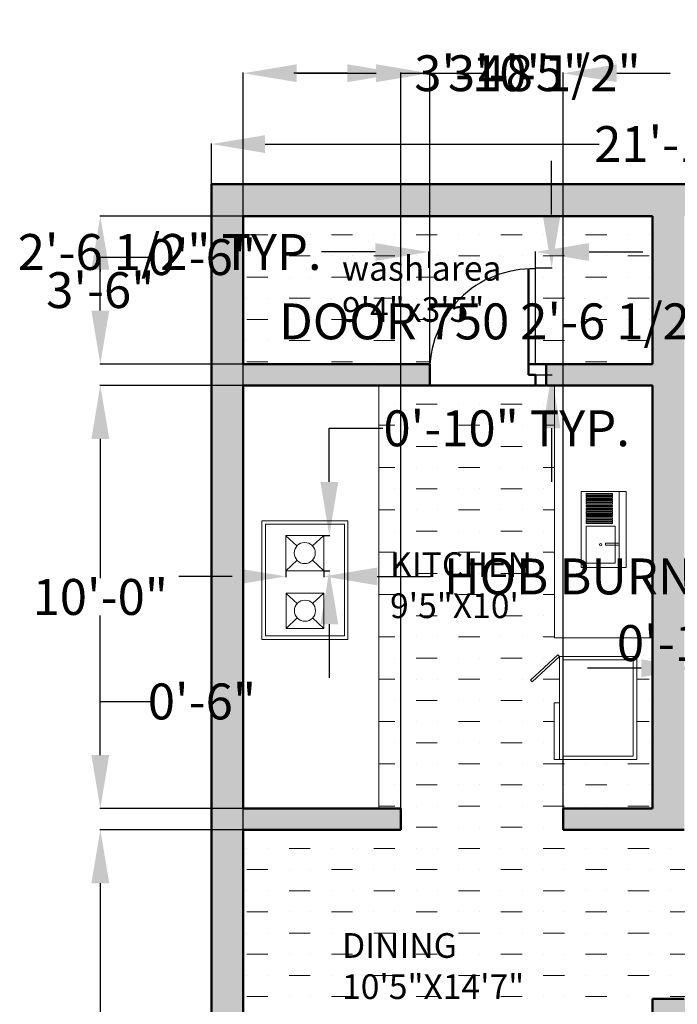
# Model space of a CAD drawing. Units: inches. Extents: x 26 to 14419, y 2 to 3479.
# Tile 4 of 9: x 13605 to 13791, y 3199 to 3479. Entities that reach past the tile are written whole.
import ezdxf

# ---------------------------------------------------------------- set-up
doc = ezdxf.new("R2010")
doc.units = ezdxf.units.IN
doc.header["$MEASUREMENT"] = 0
for name, color, linetype, lineweight in [('A-ANNO-DIMS', 2, 'Continuous', 18), ('A-AREA-IDEN', 7, 'Continuous', 18), ('A-DOOR', 4, 'Continuous', 25), ('A-FLOR-FIXT', 8, 'Continuous', 18), ('A-FLOR-PATT', 252, 'Continuous', 13), ('A-FURN', 8, 'Continuous', 18), ('A-WALL', 7, 'Continuous', 50)]:
    doc.layers.add(name, color=color, linetype=linetype, lineweight=lineweight)
doc.styles.get("Standard").update_dxf_attribs({"font": 'arial.ttf'})
doc.dimstyles.get("Standard").update_dxf_attribs({"dimtxt": 10.18, "dimasz": 15.18, "dimexe": 0.18, "dimexo": 0.0625, "dimgap": 0.09, "dimtad": 0, "dimtih": 1, "dimtoh": 1, "dimdec": 0, "dimzin": 0, "dimdsep": 46, "dimlunit": 3, "dimtxsty": 'Standard', "dimcen": 0.09, "dimadec": 0, "dimazin": 0, "dimtfac": 1, "dimtdec": 0, "dimtofl": 0, "dimtmove": 0, "dimatfit": 3, "dimfxl": 1, "dimtolj": 1, "dimtzin": 0, "dimarcsym": 0})
pattern_1 = [(0, (61.093, 57.669), (12, 6), [6, -6, 0, -6, 0, -6])]

# ---------------------------------------------------------------- blocks, each defined once
blk = doc.blocks.new('*D6')
at = {"layer": 'A-ANNO-DIMS', "color": 0, "lineweight": -2, "transparency": 16777216}
for p, q in [((13659.09, 3432.06), (13659.09, 3443.59)), ((13674.27, 3443.41), (13768.97, 3443.41)), ((13906.91, 3443.41), (13812.21, 3443.41)), ((13922.09, 3432.06), (13922.09, 3443.59))]:
    blk.add_line(p, q, dxfattribs=at)
at = {"layer": 'A-ANNO-DIMS', "color": 0, "transparency": 16777216}
for points in [[(13674.27, 3445.94), (13674.27, 3440.88), (13659.09, 3443.41)], [(13906.91, 3445.94), (13906.91, 3440.88), (13922.09, 3443.41)]]:
    blk.add_solid(points, dxfattribs=at)
at = {"layer": 'Defpoints', "color": 0, "transparency": 16777216}
for p in [(13922.09, 3443.41), (13659.09, 3432), (13922.09, 3432)]:
    blk.add_point(p, dxfattribs=at)
at = {"layer": 'A-ANNO-DIMS', "color": 0, "transparency": 16777216, "insert": (13790.59, 3443.41), "char_height": 10.18, "attachment_point": 5}
blk.add_mtext('\\A1;21\'-11"', dxfattribs=at)
blk = doc.blocks.new('DOOR-750')
blk.add_line((3, 0), (30, 0))
blk.add_arc((1, 1), 29.02, 358.0251, 91.9749)
blk = doc.blocks.new('HOB-BURNER')
for p, q in [((0, 9.87), (3.14, 7.02)), ((10.72, 10.03), (7.54, 7.06)), ((0, 0), (3.17, 2.97)), ((10.72, 0), (7.54, 2.97))]:
    blk.add_line(p, q)
blk.add_lwpolyline([(0, 10.03), (10.72, 10.03), (10.72, 0), (0, 0)], close=True)
blk.add_circle((5.36, 5.02), 2.99)
blk = doc.blocks.new('*D24')
at = {"layer": 'A-ANNO-DIMS', "color": 0, "lineweight": -2, "transparency": 16777216}
for p, q in [((13730.53, 3172.73), (13730.53, 3187.91)), ((13730.53, 3187.91), (13745.71, 3187.91)), ((13728.71, 3157.55), (13730.71, 3157.55)), ((13728.71, 3147.87), (13730.71, 3147.87)), ((13730.53, 3132.69), (13730.53, 3117.51))]:
    blk.add_line(p, q, dxfattribs=at)
at = {"layer": 'A-ANNO-DIMS', "color": 0, "transparency": 16777216}
for points in [[(13728, 3172.73), (13733.06, 3172.73), (13730.53, 3157.55)], [(13728, 3132.69), (13733.06, 3132.69), (13730.53, 3147.87)]]:
    blk.add_solid(points, dxfattribs=at)
at = {"layer": 'Defpoints', "color": 0, "transparency": 16777216}
for p in [(13728.65, 3157.55), (13730.53, 3157.55), (13728.65, 3147.87)]:
    blk.add_point(p, dxfattribs=at)
at = {"layer": 'A-ANNO-DIMS', "color": 0, "transparency": 16777216, "insert": (13788.69, 3187.91), "char_height": 10.18, "attachment_point": 5}
blk.add_mtext('\\A1;0\'-9 1/2" TYP.', dxfattribs=at)
blk = doc.blocks.new('*D27')
at = {"layer": 'A-ANNO-DIMS', "color": 0, "lineweight": -2, "transparency": 16777216}
for p, q in [((13755.48, 3423.45), (13755.48, 3438.63)), ((13751.01, 3408.27), (13755.66, 3408.27)), ((13751.01, 3378), (13755.66, 3378)), ((13755.48, 3362.82), (13755.48, 3347.64))]:
    blk.add_line(p, q, dxfattribs=at)
at = {"layer": 'A-ANNO-DIMS', "color": 0, "transparency": 16777216}
for points in [[(13752.95, 3423.45), (13758.01, 3423.45), (13755.48, 3408.27)], [(13752.95, 3362.82), (13758.01, 3362.82), (13755.48, 3378)]]:
    blk.add_solid(points, dxfattribs=at)
at = {"layer": 'Defpoints', "color": 0, "transparency": 16777216}
for p in [(13750.94, 3408.27), (13755.48, 3408.27), (13750.94, 3378)]:
    blk.add_point(p, dxfattribs=at)
at = {"layer": 'A-ANNO-DIMS', "color": 0, "transparency": 16777216, "insert": (13755.48, 3393.13), "char_height": 10.18, "attachment_point": 5}
blk.add_mtext('\\A1;DOOR 750 2\'-6 1/2" TYP.', dxfattribs=at)
blk = doc.blocks.new('*D28')
at = {"layer": 'A-ANNO-DIMS', "color": 0, "lineweight": -2, "transparency": 16777216}
for p, q in [((13705.49, 3412.81), (13690.31, 3412.81)), ((13720.67, 3408.34), (13720.67, 3412.99)), ((13750.94, 3408.34), (13750.94, 3412.99)), ((13766.12, 3412.81), (13781.3, 3412.81))]:
    blk.add_line(p, q, dxfattribs=at)
at = {"layer": 'A-ANNO-DIMS', "color": 0, "transparency": 16777216}
for points in [[(13705.49, 3415.34), (13705.49, 3410.28), (13720.67, 3412.81)], [(13766.12, 3415.34), (13766.12, 3410.28), (13750.94, 3412.81)]]:
    blk.add_solid(points, dxfattribs=at)
at = {"layer": 'Defpoints', "color": 0, "transparency": 16777216}
for p in [(13720.67, 3412.81), (13720.67, 3408.27), (13750.94, 3408.27)]:
    blk.add_point(p, dxfattribs=at)
at = {"layer": 'A-ANNO-DIMS', "color": 0, "transparency": 16777216, "insert": (13647.24, 3412.81), "char_height": 10.18, "attachment_point": 5}
blk.add_mtext('\\A1;2\'-6 1/2" TYP.', dxfattribs=at)
blk = doc.blocks.new('*D35')
at = {"layer": 'A-ANNO-DIMS', "color": 0, "lineweight": -2, "transparency": 16777216}
for p, q in [((13780.88, 3294.79), (13765.7, 3294.79)), ((13796.06, 3296.4), (13796.06, 3294.61)), ((13807.24, 3296.4), (13807.24, 3294.61)), ((13822.42, 3294.79), (13837.6, 3294.79))]:
    blk.add_line(p, q, dxfattribs=at)
at = {"layer": 'A-ANNO-DIMS', "color": 0, "transparency": 16777216}
for points in [[(13780.88, 3297.32), (13780.88, 3292.26), (13796.06, 3294.79)], [(13822.42, 3297.32), (13822.42, 3292.26), (13807.24, 3294.79)]]:
    blk.add_solid(points, dxfattribs=at)
at = {"layer": 'Defpoints', "color": 0, "transparency": 16777216}
for p in [(13796.06, 3296.46), (13807.24, 3296.46), (13807.24, 3294.79)]:
    blk.add_point(p, dxfattribs=at)
at = {"layer": 'A-ANNO-DIMS', "color": 0, "transparency": 16777216, "insert": (13893.78, 3294.79), "char_height": 10.18, "attachment_point": 5}
blk.add_mtext('\\A1;LAMP 0\'-11" TYP.', dxfattribs=at)
blk = doc.blocks.new('*D36')
at = {"layer": 'A-ANNO-DIMS', "color": 0, "lineweight": -2, "transparency": 16777216}
for p, q in [((13808.91, 3322.56), (13808.91, 3337.74)), ((13807.3, 3307.38), (13809.09, 3307.38)), ((13807.3, 3296.46), (13809.09, 3296.46)), ((13808.91, 3281.28), (13808.91, 3266.1))]:
    blk.add_line(p, q, dxfattribs=at)
at = {"layer": 'A-ANNO-DIMS', "color": 0, "transparency": 16777216}
for points in [[(13806.38, 3322.56), (13811.44, 3322.56), (13808.91, 3307.38)], [(13806.38, 3281.28), (13811.44, 3281.28), (13808.91, 3296.46)]]:
    blk.add_solid(points, dxfattribs=at)
at = {"layer": 'Defpoints', "color": 0, "transparency": 16777216}
for p in [(13807.24, 3307.38), (13808.91, 3307.38), (13807.24, 3296.46)]:
    blk.add_point(p, dxfattribs=at)
at = {"layer": 'A-ANNO-DIMS', "color": 0, "transparency": 16777216, "insert": (13808.91, 3301.92), "char_height": 10.18, "attachment_point": 5}
blk.add_mtext('\\A1;0\'-11" TYP.', dxfattribs=at)
blk = doc.blocks.new('*D47')
at = {"layer": 'A-ANNO-DIMS', "color": 0, "lineweight": -2, "transparency": 16777216}
for p, q in [((13680.17, 3322.36), (13680.17, 3320.64)), ((13690.89, 3322.36), (13690.89, 3320.64)), ((13664.99, 3320.82), (13649.81, 3320.82)), ((13706.07, 3320.82), (13721.25, 3320.82))]:
    blk.add_line(p, q, dxfattribs=at)
at = {"layer": 'A-ANNO-DIMS', "color": 0, "transparency": 16777216}
for points in [[(13664.99, 3323.35), (13664.99, 3318.29), (13680.17, 3320.82)], [(13706.07, 3323.35), (13706.07, 3318.29), (13690.89, 3320.82)]]:
    blk.add_solid(points, dxfattribs=at)
at = {"layer": 'Defpoints', "color": 0, "transparency": 16777216}
for p in [(13680.17, 3322.43), (13690.89, 3322.43), (13690.89, 3320.82)]:
    blk.add_point(p, dxfattribs=at)
at = {"layer": 'A-ANNO-DIMS', "color": 0, "transparency": 16777216, "insert": (13817.29, 3320.82), "char_height": 10.18, "attachment_point": 5}
blk.add_mtext('\\A1;HOB BURNER 0\'-10 1/2" TYP.', dxfattribs=at)
blk = doc.blocks.new('*D48')
at = {"layer": 'A-ANNO-DIMS', "color": 0, "lineweight": -2, "transparency": 16777216}
for p, q in [((13692.49, 3347.63), (13692.49, 3362.81)), ((13692.49, 3362.81), (13707.67, 3362.81)), ((13690.95, 3332.45), (13692.67, 3332.45)), ((13690.95, 3322.43), (13692.67, 3322.43)), ((13692.49, 3307.25), (13692.49, 3292.07))]:
    blk.add_line(p, q, dxfattribs=at)
at = {"layer": 'A-ANNO-DIMS', "color": 0, "transparency": 16777216}
for points in [[(13689.96, 3347.63), (13695.02, 3347.63), (13692.49, 3332.45)], [(13689.96, 3307.25), (13695.02, 3307.25), (13692.49, 3322.43)]]:
    blk.add_solid(points, dxfattribs=at)
at = {"layer": 'Defpoints', "color": 0, "transparency": 16777216}
for p in [(13690.89, 3332.45), (13692.49, 3332.45), (13690.89, 3322.43)]:
    blk.add_point(p, dxfattribs=at)
at = {"layer": 'A-ANNO-DIMS', "color": 0, "transparency": 16777216, "insert": (13742.75, 3362.81), "char_height": 10.18, "attachment_point": 5}
blk.add_mtext('\\A1;0\'-10" TYP.', dxfattribs=at)
blk = doc.blocks.new('*D58')
at = {"layer": 'A-ANNO-DIMS', "color": 0, "lineweight": -2, "transparency": 16777216}
for p, q in [((13668.03, 3249), (13627.41, 3249)), ((13627.59, 3233.82), (13627.59, 3172.29)), ((13627.59, 3100.18), (13627.59, 3161.7)), ((13668.03, 3085), (13627.41, 3085))]:
    blk.add_line(p, q, dxfattribs=at)
at = {"layer": 'A-ANNO-DIMS', "color": 0, "transparency": 16777216}
for points in [[(13625.06, 3233.82), (13630.12, 3233.82), (13627.59, 3249)], [(13625.06, 3100.18), (13630.12, 3100.18), (13627.59, 3085)]]:
    blk.add_solid(points, dxfattribs=at)
at = {"layer": 'Defpoints', "color": 0, "transparency": 16777216}
for p in [(13627.59, 3249), (13668.09, 3249), (13668.09, 3085)]:
    blk.add_point(p, dxfattribs=at)
at = {"layer": 'A-ANNO-DIMS', "color": 0, "transparency": 16777216, "insert": (13627.59, 3167), "char_height": 10.18, "attachment_point": 5}
blk.add_mtext('\\A1;13\'-8"', dxfattribs=at)
blk = doc.blocks.new('*D59')
at = {"layer": 'A-ANNO-DIMS', "color": 0, "lineweight": -2, "transparency": 16777216}
for p, q in [((13627.59, 3270.18), (13627.59, 3285.36)), ((13627.59, 3285.36), (13642.77, 3285.36)), ((13668.03, 3255), (13627.41, 3255)), ((13668.03, 3249), (13627.41, 3249)), ((13627.59, 3233.82), (13627.59, 3218.64))]:
    blk.add_line(p, q, dxfattribs=at)
at = {"layer": 'A-ANNO-DIMS', "color": 0, "transparency": 16777216}
for points in [[(13625.06, 3270.18), (13630.12, 3270.18), (13627.59, 3255)], [(13625.06, 3233.82), (13630.12, 3233.82), (13627.59, 3249)]]:
    blk.add_solid(points, dxfattribs=at)
at = {"layer": 'Defpoints', "color": 0, "transparency": 16777216}
for p in [(13627.59, 3255), (13668.09, 3255), (13668.09, 3249)]:
    blk.add_point(p, dxfattribs=at)
at = {"layer": 'A-ANNO-DIMS', "color": 0, "transparency": 16777216, "insert": (13656.39, 3285.36), "char_height": 10.18, "attachment_point": 5}
blk.add_mtext('\\A1;0\'-6"', dxfattribs=at)
blk = doc.blocks.new('*D60')
at = {"layer": 'A-ANNO-DIMS', "color": 0, "lineweight": -2, "transparency": 16777216}
for p, q in [((13668.03, 3375), (13627.41, 3375)), ((13627.59, 3359.82), (13627.59, 3320.28)), ((13627.59, 3270.18), (13627.59, 3309.71)), ((13668.03, 3255), (13627.41, 3255))]:
    blk.add_line(p, q, dxfattribs=at)
at = {"layer": 'A-ANNO-DIMS', "color": 0, "transparency": 16777216}
for points in [[(13625.06, 3359.82), (13630.12, 3359.82), (13627.59, 3375)], [(13625.06, 3270.18), (13630.12, 3270.18), (13627.59, 3255)]]:
    blk.add_solid(points, dxfattribs=at)
at = {"layer": 'Defpoints', "color": 0, "transparency": 16777216}
for p in [(13627.59, 3375), (13668.09, 3375), (13668.09, 3255)]:
    blk.add_point(p, dxfattribs=at)
at = {"layer": 'A-ANNO-DIMS', "color": 0, "transparency": 16777216, "insert": (13627.59, 3315), "char_height": 10.18, "attachment_point": 5}
blk.add_mtext('\\A1;10\'-0"', dxfattribs=at)
blk = doc.blocks.new('*D61')
at = {"layer": 'A-ANNO-DIMS', "color": 0, "lineweight": -2, "transparency": 16777216}
for p, q in [((13627.59, 3396.18), (13627.59, 3411.36)), ((13627.59, 3411.36), (13642.77, 3411.36)), ((13668.03, 3381), (13627.41, 3381)), ((13668.03, 3375), (13627.41, 3375)), ((13627.59, 3359.82), (13627.59, 3344.64))]:
    blk.add_line(p, q, dxfattribs=at)
at = {"layer": 'A-ANNO-DIMS', "color": 0, "transparency": 16777216}
for points in [[(13625.06, 3396.18), (13630.12, 3396.18), (13627.59, 3381)], [(13625.06, 3359.82), (13630.12, 3359.82), (13627.59, 3375)]]:
    blk.add_solid(points, dxfattribs=at)
at = {"layer": 'Defpoints', "color": 0, "transparency": 16777216}
for p in [(13627.59, 3381), (13668.09, 3381), (13668.09, 3375)]:
    blk.add_point(p, dxfattribs=at)
at = {"layer": 'A-ANNO-DIMS', "color": 0, "transparency": 16777216, "insert": (13656.39, 3411.36), "char_height": 10.18, "attachment_point": 5}
blk.add_mtext('\\A1;0\'-6"', dxfattribs=at)
blk = doc.blocks.new('*D62')
at = {"layer": 'A-ANNO-DIMS', "color": 0, "lineweight": -2, "transparency": 16777216}
for p, q in [((13668.03, 3423), (13627.41, 3423)), ((13627.59, 3407.82), (13627.59, 3407.29)), ((13627.59, 3396.18), (13627.59, 3396.7)), ((13668.03, 3381), (13627.41, 3381))]:
    blk.add_line(p, q, dxfattribs=at)
at = {"layer": 'A-ANNO-DIMS', "color": 0, "transparency": 16777216}
for points in [[(13625.06, 3407.82), (13630.12, 3407.82), (13627.59, 3423)], [(13625.06, 3396.18), (13630.12, 3396.18), (13627.59, 3381)]]:
    blk.add_solid(points, dxfattribs=at)
at = {"layer": 'Defpoints', "color": 0, "transparency": 16777216}
for p in [(13627.59, 3423), (13668.09, 3423), (13668.09, 3381)]:
    blk.add_point(p, dxfattribs=at)
at = {"layer": 'A-ANNO-DIMS', "color": 0, "transparency": 16777216, "insert": (13627.59, 3402), "char_height": 10.18, "attachment_point": 5}
blk.add_mtext('\\A1;3\'-6"', dxfattribs=at)
blk = doc.blocks.new('*D75')
at = {"layer": 'A-ANNO-DIMS', "color": 0, "lineweight": -2, "transparency": 16777216}
for p, q in [((13668.09, 3249.06), (13668.09, 3463.68)), ((13683.27, 3463.5), (13697.58, 3463.5)), ((13712.76, 3249.06), (13712.76, 3463.68)), ((13712.76, 3463.5), (13727.94, 3463.5))]:
    blk.add_line(p, q, dxfattribs=at)
at = {"layer": 'A-ANNO-DIMS', "color": 0, "transparency": 16777216}
for points in [[(13683.27, 3466.03), (13683.27, 3460.97), (13668.09, 3463.5)], [(13697.58, 3466.03), (13697.58, 3460.97), (13712.76, 3463.5)]]:
    blk.add_solid(points, dxfattribs=at)
at = {"layer": 'Defpoints', "color": 0, "transparency": 16777216}
for p in [(13712.76, 3463.5), (13668.09, 3249), (13712.76, 3249)]:
    blk.add_point(p, dxfattribs=at)
at = {"layer": 'A-ANNO-DIMS', "color": 0, "transparency": 16777216, "insert": (13753.42, 3463.5), "char_height": 10.18, "attachment_point": 5}
blk.add_mtext('\\A1;3\'-8 1/2"', dxfattribs=at)
blk = doc.blocks.new('*D76')
at = {"layer": 'A-ANNO-DIMS', "color": 0, "lineweight": -2, "transparency": 16777216}
for p, q in [((13697.580042, 3463.496029), (13682.400042, 3463.496029)), ((13712.760042, 3249.058529), (13712.760042, 3463.676029)), ((13758.766114, 3249.058529), (13758.766114, 3463.676029)), ((13773.946114, 3463.496029), (13789.126114, 3463.496029))]:
    blk.add_line(p, q, dxfattribs=at)
at = {"layer": 'A-ANNO-DIMS', "color": 0, "transparency": 16777216}
for points in [[(13697.580042, 3466.026029), (13697.580042, 3460.966029), (13712.760042, 3463.496029)], [(13773.946114, 3466.026029), (13773.946114, 3460.966029), (13758.766114, 3463.496029)]]:
    blk.add_solid(points, dxfattribs=at)
at = {"layer": 'Defpoints', "color": 0, "transparency": 16777216}
for p in [(13758.766114, 3463.496029), (13712.760042, 3248.996029), (13758.766114, 3248.996029)]:
    blk.add_point(p, dxfattribs=at)
at = {"layer": 'A-ANNO-DIMS', "color": 0, "transparency": 16777216, "insert": (13735.763078, 3463.496029), "char_height": 10.18, "attachment_point": 5}
blk.add_mtext('\\A1;3\'-10"', dxfattribs=at)
blk = doc.blocks.new('*D77')
at = {"layer": 'A-ANNO-DIMS', "color": 0, "lineweight": -2, "transparency": 16777216}
for p, q in [((13668.09, 3381.06), (13668.09, 3463.68)), ((13683.27, 3463.5), (13705.76, 3463.5)), ((13720.94, 3381.06), (13720.94, 3463.68)), ((13720.94, 3463.5), (13736.12, 3463.5))]:
    blk.add_line(p, q, dxfattribs=at)
at = {"layer": 'A-ANNO-DIMS', "color": 0, "transparency": 16777216}
for points in [[(13683.27, 3466.03), (13683.27, 3460.97), (13668.09, 3463.5)], [(13705.76, 3466.03), (13705.76, 3460.97), (13720.94, 3463.5)]]:
    blk.add_solid(points, dxfattribs=at)
at = {"layer": 'Defpoints', "color": 0, "transparency": 16777216}
for p in [(13720.94, 3463.5), (13668.09, 3381), (13720.94, 3381)]:
    blk.add_point(p, dxfattribs=at)
at = {"layer": 'A-ANNO-DIMS', "color": 0, "transparency": 16777216, "insert": (13749.95, 3463.5), "char_height": 10.18, "attachment_point": 5}
blk.add_mtext('\\A1;4\'-5"', dxfattribs=at)

msp = doc.modelspace()

# ---------------------------------------------------------------- hatches: boundary and pattern name
at = {"layer": 'A-FLOR-PATT'}
h = msp.add_hatch(color=256, dxfattribs=at)
h.dxf.hatch_style = 1
h.paths.add_polyline_path([(13922.09, 3432), (13659.09, 3432), (13659.09, 2842), (13668.09, 2842), (13668.09, 2851), (13668.09, 2899), (13668.09, 2908), (13668.09, 3076), (13706.09, 3076), (13706.09, 3085), (13668.09, 3085), (13668.09, 3249), (13712.76, 3249), (13712.76, 3255), (13668.09, 3255), (13668.09, 3375), (13720.94, 3375), (13720.94, 3378, -0.017236), (13720.94, 3380), (13720.94, 3381), (13668.09, 3381), (13668.09, 3423), (13784.09, 3423), (13784.09, 3381), (13753.94, 3381), (13753.94, 3375), (13784.09, 3375), (13784.09, 3255), (13758.77, 3255), (13758.77, 3249), (13784.09, 3249), (13793.09, 3249), (13793.09, 3255), (13793.09, 3423), (13913.09, 3423), (13913.09, 3255), (13832.09, 3255), (13832.09, 3254, -0.014283), (13832.09, 3252), (13832.09, 3249), (13836.57, 3249), (13836.57, 3234), (13839.57, 3234, -0.017236), (13841.57, 3234), (13842.57, 3234), (13842.57, 3249), (13913.09, 3249), (13913.09, 3201), (13892.46, 3201), (13793.09, 3201), (13784.09, 3201), (13784.09, 3195), (13793.09, 3195), (13913.09, 3195), (13913.09, 3127), (13922.09, 3127)])
h.paths.add_polyline_path([(13922.09, 3013.5), (13913.09, 3013.5), (13913.09, 2908), (13892.09, 2908), (13892.09, 2899), (13913.09, 2899), (13913.09, 2851), (13793.09, 2851), (13784.09, 2851), (13784.09, 2842), (13922.09, 2842)], flags=17)
h.paths.add_polyline_path([(13793.09, 3085), (13784.09, 3085), (13784.09, 3076), (13784.09, 3071.08), (13784.09, 3066.17), (13784.09, 2908), (13784.09, 2899.07), (13793.09, 2899), (13802.09, 2899), (13814.09, 2899), (13814.09, 2908), (13793.09, 2908)], flags=17)
h.paths.add_polyline_path([(14342.64, 3401.72), (14242.78, 3401.72), (14242.78, 3392.72), (14257.64, 3392.72), (14257.64, 3351.75), (14257.64, 3345.75), (14257.64, 3330.73), (14263.64, 3330.73), (14263.64, 3392.72), (14333.64, 3392.72), (14333.64, 3284.72), (14302.92, 3284.72), (14302.92, 3281.72, -0.022645), (14302.92, 3279.12), (14302.92, 3278.72), (14333.64, 3278.72), (14333.64, 3170.72), (14316.1, 3170.72), (14263.64, 3170.72), (14263.64, 3278.72), (14269.92, 3278.72), (14269.92, 3284.72), (14263.64, 3284.72), (14257.64, 3284.72), (14257.64, 3225.75), (14257.64, 3219.75), (14257.64, 3164.72), (14333.64, 3164.72), (14333.64, 3110.37), (14210.01, 3110.37), (14210.01, 3104.37), (14257.64, 3104.37), (14257.64, 3024), (14263.64, 3024), (14263.64, 3039.72), (14263.64, 3104.37), (14333.64, 3104.37), (14333.64, 3045.72), (14333.64, 3039.72), (14333.64, 2967.72), (14296.64, 2967.72), (14296.64, 2964.72, -0.017236), (14296.64, 2962.72), (14296.64, 2961.72), (14333.64, 2961.72), (14333.64, 2882.72), (14312.64, 2882.72), (14312.64, 2873.72), (14333.64, 2873.72), (14333.64, 2820.72), (14333.64, 2811.72), (14342.64, 2811.72)])
h.paths.add_polyline_path([(14088.64, 3219.75), (14218.64, 3219.75), (14218.64, 3222.75, -0.014283), (14218.64, 3224.75), (14218.64, 3225.75), (14088.64, 3225.75), (14088.64, 3345.75), (14088.64, 3351.75), (14088.64, 3392.72), (14193.93, 3392.72), (14193.93, 3351.75), (14140.64, 3351.75), (14140.64, 3345.75), (14170.7, 3345.75), (14218.64, 3345.75), (14218.64, 3348.75, -0.014283), (14218.64, 3350.75), (14218.64, 3351.75), (14199.93, 3351.75), (14199.93, 3392.72), (14214.78, 3392.72), (14214.78, 3401.72), (14079.64, 3401.72), (14079.64, 2811.72), (14088.64, 2811.72), (14088.64, 2820.72), (14088.64, 2873.72), (14116.21, 2873.72), (14116.21, 2876.57), (14116.21, 2882.72), (14088.64, 2882.72), (14088.64, 3039.72), (14216.01, 3039.72), (14216.01, 3065.37), (14215.01, 3065.37, -0.014283), (14213.01, 3065.37), (14210.01, 3065.37), (14210.01, 3045.72), (14154.64, 3045.72), (14148.64, 3045.72), (14088.64, 3045.72)])
h.paths.add_polyline_path([(14284.64, 2882.72), (14263.64, 2882.72), (14263.64, 2961.72), (14263.64, 2967.72), (14257.64, 2967.72), (14257.64, 2956.69), (14257.64, 2916.18), (14257.64, 2882.72), (14249.61, 2882.72), (14249.61, 2873.72), (14284.64, 2873.72)], flags=17)
h.paths.add_polyline_path([(14202.78, 2882.72), (14189.55, 2882.72), (14189.55, 2879.95), (14189.55, 2873.72), (14202.78, 2873.72)], flags=17)
h = msp.add_hatch(dxfattribs=at)
h.set_pattern_fill('MUDST', color=256, scale=24)
h.set_pattern_definition(pattern_1)
h.paths.add_polyline_path([(13720.99, 3381, -0.404142), (13750.94, 3408), (13750.94, 3381), (13784.09, 3381), (13784.09, 3423), (13668.09, 3423), (13668.09, 3381)])
h = msp.add_hatch(dxfattribs=at)
h.set_pattern_fill('MUDST', color=256, scale=24)
h.set_pattern_definition(pattern_1)
h.paths.add_polyline_path([(13756.28, 3375), (13750.94, 3375), (13720.94, 3375), (13706.54, 3375), (13706.54, 3255), (13712.76, 3255), (13712.76, 3249), (13668.09, 3249), (13668.09, 3085), (13709.09, 3085), (13709.09, 3116.5, -0.393405), (13744.93, 3085), (13745.25, 3085, -0.393405), (13781.09, 3116.5), (13781.09, 3085), (13784.09, 3085), (13784.09, 3127), (13784.09, 3195), (13784.09, 3201), (13793.09, 3201), (13836.57, 3201), (13836.57, 3204), (13836.57, 3234), (13836.57, 3249), (13832.09, 3249), (13832.09, 3254, 0.397579), (13798.09, 3288), (13798.09, 3252), (13796.09, 3252), (13796.09, 3249), (13793.09, 3249), (13784.09, 3249), (13758.77, 3249), (13758.77, 3255), (13784.09, 3255), (13784.09, 3303.43), (13756.28, 3303.43)])
h.paths.add_polyline_path([(13757.29, 3298.63), (13757.76, 3298.12), (13779.63, 3298.12), (13779.63, 3268.87), (13757.77, 3268.87), (13756.19, 3268.87), (13756.19, 3285.02), (13757.77, 3285.02), (13757.77, 3298.11), (13749.96, 3290.89), (13749.48, 3291.4)], flags=16)
h.paths.add_polyline_path([(13758.77, 3297.12), (13778.63, 3297.12), (13778.63, 3269.87), (13758.77, 3269.87)], flags=0)
h.paths.add_polyline_path([(13716.08, 3198.11), (13716.08, 3190.37), (13728.65, 3190.37), (13728.65, 3180.68), (13716.08, 3180.68), (13716.08, 3174.63), (13728.65, 3174.63), (13728.65, 3164.95), (13716.08, 3164.95), (13716.08, 3157.55), (13728.65, 3157.55), (13728.65, 3147.87), (13716.08, 3147.87), (13716.08, 3142.39), (13687.89, 3142.39), (13687.89, 3145.78), (13675.33, 3145.78), (13675.33, 3155.46), (13687.89, 3155.46), (13687.89, 3163.27), (13675.33, 3163.27), (13675.33, 3172.95), (13687.89, 3172.95), (13687.89, 3179.58), (13675.33, 3179.58), (13675.33, 3189.26), (13687.89, 3189.26), (13687.89, 3198.11)], flags=16)
h.paths.add_polyline_path([(13715.08, 3197.11), (13715.08, 3143.39), (13688.89, 3143.39), (13688.89, 3197.11)], flags=0)

# ---------------------------------------------------------------- linework, layer by layer
at = {"layer": 'A-FLOR-FIXT'}
for p, q in [((13756.28, 3375), (13756.28, 3303.43)), ((13774.68, 3344.9), (13774.68, 3323.37)), ((13756.28, 3303.43), (13784.09, 3303.43))]:
    msp.add_line(p, q, dxfattribs=at)
for points in [[(13763.89, 3344.9), (13776.66, 3344.9), (13776.66, 3323.37), (13763.89, 3323.37)], [(13765.26, 3344.3), (13772.79, 3344.3), (13772.79, 3343.96), (13765.26, 3343.96)], [(13765.26, 3343.88), (13772.79, 3343.88), (13772.79, 3343.54), (13765.26, 3343.54)], [(13765.26, 3343.35), (13772.79, 3343.35), (13772.79, 3343.01), (13765.26, 3343.01)], [(13765.26, 3342.76), (13772.79, 3342.76), (13772.79, 3342.42), (13765.26, 3342.42)], [(13765.26, 3342.21), (13772.79, 3342.21), (13772.79, 3341.87), (13765.26, 3341.87)], [(13765.26, 3341.64), (13772.79, 3341.64), (13772.79, 3341.3), (13765.26, 3341.3)], [(13765.26, 3340.97), (13772.79, 3340.97), (13772.79, 3340.63), (13765.26, 3340.63)], [(13765.26, 3340.29), (13772.79, 3340.29), (13772.79, 3339.95), (13765.26, 3339.95)], [(13765.26, 3339.75), (13772.79, 3339.75), (13772.79, 3339.41), (13765.26, 3339.41)], [(13765.26, 3339.1), (13772.79, 3339.1), (13772.79, 3338.76), (13765.26, 3338.76)], [(13673.41, 3336.62), (13697.76, 3336.62), (13697.76, 3302.97), (13673.41, 3302.97)], [(13765.25, 3338.68), (13772.78, 3338.68), (13772.78, 3338.34), (13765.25, 3338.34)], [(13765.26, 3338.12), (13772.79, 3338.12), (13772.79, 3337.79), (13765.26, 3337.79)], [(13765.26, 3337.43), (13772.79, 3337.43), (13772.79, 3337.09), (13765.26, 3337.09)], [(13765.26, 3336.73), (13772.79, 3336.73), (13772.79, 3336.39), (13765.26, 3336.39)], [(13674.41, 3335.62), (13696.76, 3335.62), (13696.76, 3303.97), (13674.41, 3303.97)], [(13765.26, 3336.21), (13772.79, 3336.21), (13772.79, 3335.87), (13765.26, 3335.87)], [(13765.29, 3335.05), (13773.54, 3335.05), (13773.54, 3324.58), (13765.29, 3324.58)], [(13774.68, 3330.29), (13770.8, 3330.29), (13770.8, 3329.69), (13774.68, 3329.69)], [(13749.48, 3291.4), (13757.29, 3298.63), (13757.77, 3298.11), (13749.96, 3290.89)], [(13779.63, 3298.12), (13757.77, 3298.12), (13757.77, 3268.87), (13779.63, 3268.87)], [(13778.63, 3297.12), (13758.77, 3297.12), (13758.77, 3269.87), (13778.63, 3269.87)], [(13757.77, 3268.87), (13756.19, 3268.87), (13756.19, 3285.02), (13757.77, 3285.02)]]:
    msp.add_lwpolyline(points, close=True, dxfattribs=at)
msp.add_circle((13769.41, 3329.82), 0.353, dxfattribs=at)
at = {"layer": 'A-FURN'}
msp.add_line((13706.54, 3375), (13706.54, 3255), dxfattribs=at)
at = {"layer": 'A-WALL'}
for p, q in [((13659.09, 2842), (13659.09, 3432)), ((13659.09, 3432), (13922.09, 3432)), ((13668.09, 3423), (13784.09, 3423)), ((13668.09, 3381), (13668.09, 3423)), ((13784.09, 3381), (13784.09, 3423)), ((13748.94, 3378), (13748.94, 3408)), ((13668.09, 3381), (13720.99, 3381)), ((13720.94, 3381), (13720.94, 3375)), ((13748.94, 3381), (13784.09, 3381)), ((13753.94, 3381), (13753.94, 3375)), ((13748.94, 3378), (13750.94, 3378)), ((13750.94, 3378), (13750.94, 3375)), ((13668.09, 3375), (13720.94, 3375)), ((13668.09, 3255), (13668.09, 3375)), ((13720.94, 3375), (13750.94, 3375)), ((13750.94, 3375), (13784.09, 3375)), ((13784.09, 3255), (13784.09, 3375)), ((13668.09, 3255), (13712.76, 3255)), ((13712.76, 3255), (13712.76, 3249)), ((13758.77, 3255), (13758.77, 3249)), ((13758.77, 3255), (13784.09, 3255)), ((13668.09, 3249), (13712.76, 3249)), ((13668.09, 3085), (13668.09, 3249)), ((13758.77, 3249), (13784.09, 3249)), ((13784.09, 3249), (13793.09, 3249)), ((13784.09, 3195), (13784.09, 3201)), ((13793.09, 3201), (13784.09, 3201))]:
    msp.add_line(p, q, dxfattribs=at)

# ---------------------------------------------------------------- block references
at = {"layer": 'A-DOOR', "rotation": 89.99999999999655}
msp.add_blockref('DOOR-750', (13750.94, 3378), dxfattribs=at)
at = {"layer": 'A-FLOR-FIXT'}
for p in [(13680.17, 3322.43), (13680.23, 3306.08)]:
    msp.add_blockref('HOB-BURNER', p, dxfattribs=at)

# ---------------------------------------------------------------- texts
at = {"layer": 'A-AREA-IDEN', "char_height": 7, "attachment_point": 1}
for s, insert in [('wash area\\P9\'4"x3\'5"', (13696.09, 3411.67)), ('KITCHEN\\P9\'5"X10\'', (13709.7, 3327.67)), ('DINING\\P10\'5"X14\'7"', (13696.09, 3219.67))]:
    msp.add_mtext_dynamic_manual_height_columns(s, width=51, gutter_width=1, heights=[0], dxfattribs=dict(at, insert=insert))

# ---------------------------------------------------------------- dimensions: what is measured, and where the dimension line sits
at = {"layer": 'A-ANNO-DIMS'}
for base, p1, p2, override, picture, middle in [((13712.76, 3463.5), (13668.09, 3249), (13712.76, 3249), {"dimdec": 1, "dimlfac": 1, "dimrnd": 0, "dimzin": 1, "dimdsep": 46, "dimlunit": 4, "dimfrac": 2}, '*D75', (13753.42, 3463.5)), ((13720.9431, 3463.496), (13668.0912, 3380.996), (13720.9431, 3380.996), {"dimdec": 1, "dimlfac": 1, "dimrnd": 0, "dimzin": 1, "dimdsep": 46, "dimlunit": 4, "dimfrac": 2}, '*D77', (13749.9485, 3463.496)), ((13758.77, 3463.5), (13712.76, 3249), (13758.77, 3249), {"dimdec": 1, "dimlfac": 1, "dimrnd": 0, "dimzin": 1, "dimdsep": 46, "dimlunit": 4, "dimfrac": 2}, '*D76', (13735.76, 3463.5)), ((13922.09, 3443.41), (13659.09, 3432), (13922.09, 3432), {"dimclrd": 0, "dimclre": 0, "dimclrt": 0}, '*D6', (13790.59, 3443.41))]:
    dim = msp.add_linear_dim(base=base, p1=p1, p2=p2, dimstyle='Standard', override=override, dxfattribs=at)
    dim.commit()
    dim.dimension.update_dxf_attribs({"geometry": picture, "text_midpoint": middle})
for base, p1, p2, angle, text, picture, middle in [((13755.48, 3408.27), (13750.94, 3378), (13750.94, 3408.27), 90, 'DOOR 750 <> TYP.', '*D27', (13755.48, 3393.13)), ((13720.67, 3412.81), (13750.94, 3408.27), (13720.67, 3408.27), 180, '<> TYP.', '*D28', (13647.24, 3412.81)), ((13692.49, 3332.45), (13690.89, 3322.43), (13690.89, 3332.45), 90, '<> TYP.', '*D48', (13742.75, 3362.81)), ((13808.91, 3307.38), (13807.24, 3296.46), (13807.24, 3307.38), 90, '<> TYP.', '*D36', (13808.91, 3301.92)), ((13730.53, 3157.55), (13728.65, 3147.87), (13728.65, 3157.55), 90, '<> TYP.', '*D24', (13788.69, 3187.91))]:
    dim = msp.add_linear_dim(base=base, p1=p1, p2=p2, angle=angle, text=text, dimstyle='Standard', override={"dimdec": 1, "dimrnd": 0, "dimzin": 1, "dimlunit": 4, "dimfrac": 2}, dxfattribs=at)
    dim.commit()
    dim.dimension.update_dxf_attribs({"geometry": picture, "text_midpoint": middle})
for base, p1, p2, picture, middle in [((13627.59, 3423), (13668.09, 3381), (13668.09, 3423), '*D62', (13627.59, 3402)), ((13627.59, 3381), (13668.09, 3375), (13668.09, 3381), '*D61', (13656.39, 3411.36)), ((13627.59, 3375), (13668.09, 3255), (13668.09, 3375), '*D60', (13627.59, 3315)), ((13627.59, 3255), (13668.09, 3249), (13668.09, 3255), '*D59', (13656.39, 3285.36)), ((13627.59, 3249), (13668.09, 3085), (13668.09, 3249), '*D58', (13627.59, 3167))]:
    dim = msp.add_linear_dim(base=base, p1=p1, p2=p2, angle=90, dimstyle='Standard', override={"dimdec": 1, "dimlfac": 1, "dimrnd": 0, "dimzin": 1, "dimdsep": 46, "dimlunit": 4, "dimfrac": 2}, dxfattribs=at)
    dim.commit()
    dim.dimension.update_dxf_attribs({"geometry": picture, "text_midpoint": middle})
for base, p1, p2, text, picture, middle in [((13690.89, 3320.82), (13680.17, 3322.43), (13690.89, 3322.43), 'HOB BURNER <> TYP.', '*D47', (13817.29, 3320.82)), ((13807.24, 3294.79), (13796.06, 3296.46), (13807.24, 3296.46), 'LAMP <> TYP.', '*D35', (13893.78, 3294.79))]:
    dim = msp.add_linear_dim(base=base, p1=p1, p2=p2, text=text, dimstyle='Standard', override={"dimdec": 1, "dimrnd": 0, "dimzin": 1, "dimlunit": 4, "dimfrac": 2}, dxfattribs=at)
    dim.commit()
    dim.dimension.update_dxf_attribs({"geometry": picture, "text_midpoint": middle})

doc.saveas('drawing.dxf')
